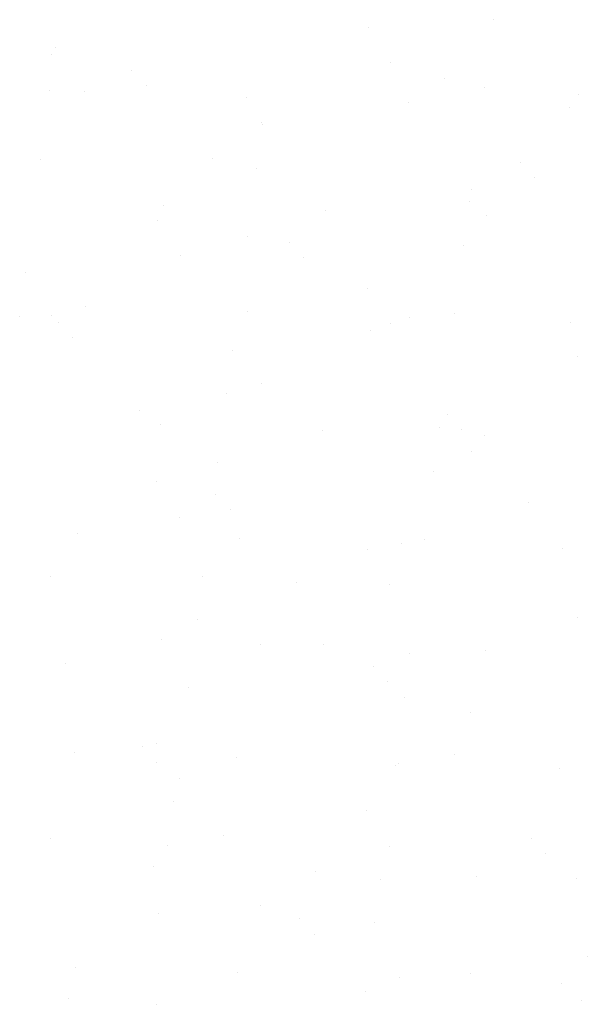
# Model space of a CAD drawing. Units: millimetres. Extents: x -857 to 54106, y -13666 to 13947.
# Tile 34 of 41: x 31165 to 31471, y 9454 to 9984. Entities that reach past the tile are written whole.
import ezdxf

# ---------------------------------------------------------------- set-up
doc = ezdxf.new("R2010")
doc.units = ezdxf.units.MM
doc.layers.add('A-FURN', color=21, linetype='Continuous', lineweight=18)
doc.layers.add('A-HT', color=15, linetype='Continuous')

# ---------------------------------------------------------------- blocks, each defined once
blk = doc.blocks.new('*X18')
at = {"color": 0}
for p, q in [((1.92444, 2.71305), (1.92444, 2.71305)), ((1.95047, 2.71648), (1.95047, 2.71648)), ((1.85653, 2.70411), (1.85653, 2.70411)), ((1.78985, 2.69533), (1.78985, 2.69533)), ((1.79412, 2.69753), (1.79412, 2.69753)), ((1.81588, 2.69876), (1.81588, 2.69876)), ((1.94983, 2.69782), (1.94983, 2.69782)), ((2.10553, 2.6981), (2.10553, 2.6981)), ((2.26124, 2.69838), (2.26124, 2.69838)), ((1.95397, 2.69351), (1.95397, 2.69351)), ((2.15699, 2.68909), (2.15699, 2.68909)), ((1.96319, 2.68507), (1.96319, 2.68507)), ((2.07944, 2.68195), (2.07944, 2.68195)), ((2.21032, 2.68362), (2.21032, 2.68362)), ((2.33823, 2.68301), (2.33823, 2.68301)), ((2.35707, 2.68737), (2.35707, 2.68737)), ((1.81649, 2.6777), (1.81649, 2.6777)), ((1.9444, 2.67708), (1.9444, 2.67708)), ((1.80367, 2.64963), (1.80367, 2.64963)), ((1.81288, 2.64119), (1.81288, 2.64119)), ((2.00669, 2.64521), (2.00669, 2.64521)), ((2.20676, 2.64349), (2.20676, 2.64349)), ((2.20463, 2.63497), (2.20463, 2.63497)), ((2.21598, 2.63505), (2.21598, 2.63505)), ((2.27793, 2.63674), (2.27793, 2.63674)), ((2.36034, 2.63525), (2.36034, 2.63525)), ((1.8841, 2.63082), (1.8841, 2.63082)), ((1.89322, 2.6344), (1.89322, 2.6344)), ((2.01498, 2.63249), (2.01498, 2.63249)), ((2.04892, 2.63468), (2.04892, 2.63468)), ((2.14289, 2.63187), (2.14289, 2.63187)), ((2.30639, 2.63388), (2.30639, 2.63388)), ((2.23972, 2.6251), (2.23972, 2.6251)), ((2.26574, 2.62853), (2.26574, 2.62853)), ((1.9143, 2.62097), (1.9143, 2.62097)), ((2.07001, 2.62125), (2.07001, 2.62125)), ((2.22572, 2.62153), (2.22572, 2.62153)), ((2.1718, 2.61616), (2.1718, 2.61616)), ((2.10513, 2.60738), (2.10513, 2.60738)), ((2.13115, 2.61081), (2.13115, 2.61081)), ((1.85638, 2.60133), (1.85638, 2.60133)), ((2.03721, 2.59844), (2.03721, 2.59844)), ((2.05645, 2.59961), (2.05645, 2.59961)), ((2.25948, 2.59519), (2.25948, 2.59519)), ((1.97054, 2.58966), (1.97054, 2.58966)), ((1.99656, 2.59309), (1.99656, 2.59309)), ((2.06567, 2.59116), (2.06567, 2.59116)), ((2.08259, 2.58561), (2.08259, 2.58561)), ((2.21347, 2.58728), (2.21347, 2.58728)), ((2.34138, 2.58666), (2.34138, 2.58666)), ((1.81964, 2.58136), (1.81964, 2.58136)), ((1.90263, 2.58072), (1.90263, 2.58072)), ((1.94755, 2.58074), (1.94755, 2.58074)), ((1.8345, 2.57233), (1.8345, 2.57233)), ((1.83595, 2.57194), (1.83595, 2.57194)), ((1.86198, 2.57537), (1.86198, 2.57537)), ((1.99021, 2.57261), (1.99021, 2.57261)), ((2.14592, 2.57289), (2.14592, 2.57289)), ((2.30162, 2.57318), (2.30162, 2.57318)), ((1.90615, 2.55572), (1.90615, 2.55572)), ((1.91536, 2.54728), (1.91536, 2.54728)), ((2.10917, 2.5513), (2.10917, 2.5513)), ((2.30924, 2.54958), (2.30924, 2.54958)), ((2.31846, 2.54114), (2.31846, 2.54114)), ((2.01813, 2.53615), (2.01813, 2.53615)), ((2.14604, 2.53553), (2.14604, 2.53553)), ((2.28108, 2.5404), (2.28108, 2.5404)), ((1.88725, 2.53448), (1.88725, 2.53448)), ((1.77789, 2.50891), (1.77789, 2.50891)), ((1.9336, 2.5092), (1.9336, 2.5092)), ((1.95886, 2.50742), (1.95886, 2.50742)), ((2.08931, 2.50948), (2.08931, 2.50948)), ((2.24501, 2.50976), (2.24501, 2.50976)), ((2.35249, 2.51049), (2.35249, 2.51049)), ((2.15894, 2.5057), (2.15894, 2.5057)), ((2.28582, 2.50171), (2.28582, 2.50171)), ((2.31184, 2.50514), (2.31184, 2.50514)), ((1.79898, 2.49548), (1.79898, 2.49548)), ((1.95468, 2.49576), (1.95468, 2.49576)), ((2.11039, 2.49605), (2.11039, 2.49605)), ((2.16815, 2.49726), (2.16815, 2.49726)), ((2.2661, 2.49633), (2.2661, 2.49633)), ((2.08574, 2.48927), (2.08574, 2.48927)), ((2.21662, 2.49094), (2.21662, 2.49094)), ((2.2179, 2.49277), (2.2179, 2.49277)), ((2.34453, 2.49032), (2.34453, 2.49032)), ((1.82279, 2.48502), (1.82279, 2.48502)), ((1.9507, 2.4844), (1.9507, 2.4844)), ((2.15123, 2.48399), (2.15123, 2.48399)), ((2.17725, 2.48742), (2.17725, 2.48742)), ((2.08331, 2.47505), (2.08331, 2.47505)), ((2.01664, 2.46627), (2.01664, 2.46627)), ((2.04266, 2.4697), (2.04266, 2.4697)), ((1.80856, 2.46353), (1.80856, 2.46353)), ((2.00863, 2.46182), (2.00863, 2.46182)), ((1.94873, 2.45733), (1.94873, 2.45733)), ((2.01784, 2.45337), (2.01784, 2.45337)), ((2.21165, 2.4574), (2.21165, 2.4574)), ((1.88205, 2.44855), (1.88205, 2.44855)), ((1.90808, 2.45198), (1.90808, 2.45198)), ((2.03059, 2.44741), (2.03059, 2.44741)), ((2.1863, 2.44769), (2.1863, 2.44769)), ((2.342, 2.44797), (2.342, 2.44797)), ((1.87488, 2.44712), (1.87488, 2.44712)), ((2.28423, 2.44406), (2.28423, 2.44406)), ((1.81414, 2.43961), (1.81414, 2.43961)), ((1.8904, 2.43814), (1.8904, 2.43814)), ((2.02128, 2.43981), (2.02128, 2.43981)), ((2.14919, 2.43919), (2.14919, 2.43919)), ((1.77349, 2.43426), (1.77349, 2.43426)), ((1.85832, 2.41793), (1.85832, 2.41793)), ((2.06134, 2.41351), (2.06134, 2.41351)), ((1.86754, 2.40949), (1.86754, 2.40949)), ((2.26142, 2.41179), (2.26142, 2.41179)), ((2.27063, 2.40335), (2.27063, 2.40335)), ((2.21977, 2.3946), (2.21977, 2.3946)), ((1.82594, 2.38867), (1.82594, 2.38867)), ((2.08889, 2.39293), (2.08889, 2.39293)), ((2.34768, 2.39398), (2.34768, 2.39398)), ((1.81827, 2.38371), (1.81827, 2.38371)), ((1.95385, 2.38806), (1.95385, 2.38806)), ((1.97398, 2.38399), (1.97398, 2.38399)), ((2.12969, 2.38427), (2.12969, 2.38427)), ((2.28539, 2.38456), (2.28539, 2.38456)), ((2.33192, 2.37832), (2.33192, 2.37832)), ((2.35794, 2.38175), (2.35794, 2.38175))]:
    blk.add_line(p, q, dxfattribs=at)
blk = doc.blocks.new('A$C6796526C')
at = {"layer": 'A-HT', "extrusion": (0, 0, -1), "zscale": -1, "rotation": 180}
blk.add_blockref('*X18', (0.55, 3), dxfattribs=at)

msp = doc.modelspace()

# ---------------------------------------------------------------- block references
at = {"layer": 'A-FURN', "xscale": 903.6084929786902, "yscale": 903.6084929786902, "zscale": 903.6084929786902, "rotation": 269.9999999999988}
msp.add_blockref('A$C6796526C', (30909.253, 11089.463), dxfattribs=at)

doc.saveas('drawing.dxf')
